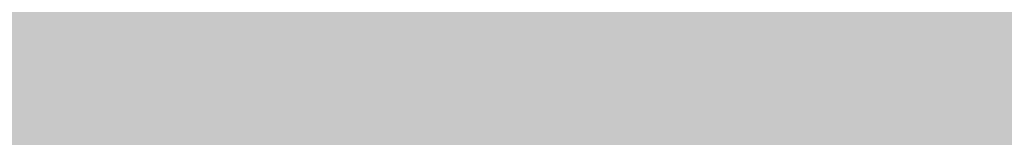
# Model space of a CAD drawing. Units: millimetres. Extents: x 0 to 2267, y 0 to 1823.
# Tile 203 of 256: x 1841.442 to 1842.748, y 1127.15 to 1127.306. Entities that reach past the tile are written whole.
import ezdxf

# ---------------------------------------------------------------- set-up
doc = ezdxf.new("R2010")
doc.units = ezdxf.units.MM
doc.header["$MEASUREMENT"] = 0
doc.layers.add('M-DIMS', color=2, linetype='Continuous', lineweight=25)
doc.layers.add('M-HATC', color=252, linetype='Continuous', lineweight=18)
doc.styles.get("Standard").update_dxf_attribs({"font": 'arial.ttf'})
doc.dimstyles.get("Standard").update_dxf_attribs({"dimtxt": 7, "dimasz": 4, "dimexe": 0.18, "dimexo": 0.0625, "dimgap": 0.09, "dimtad": 0, "dimdec": 0, "dimzin": 0, "dimdsep": 46, "dimtxsty": 'Standard', "dimcen": 0.09, "dimadec": 0, "dimazin": 0, "dimtfac": 1, "dimtdec": 0, "dimtofl": 0, "dimtmove": 0, "dimatfit": 3, "dimfxl": 1, "dimtolj": 1, "dimtzin": 0, "dimarcsym": 0})

# ---------------------------------------------------------------- blocks, each defined once
blk = doc.blocks.new('*D1')
at = {"layer": 'Defpoints', "color": 0, "transparency": 16777216}
for p in [(1593.4289, 1127.4171), (1843.4289, 1127.4171), (1843.4289, 955.6278)]:
    blk.add_point(p, dxfattribs=at)
at = {"layer": 'M-DIMS', "color": 0, "lineweight": -2, "transparency": 16777216}
for p, q in [((1593.4289, 1127.3546), (1593.4289, 955.4478)), ((1843.4289, 1127.3546), (1843.4289, 955.4478)), ((1597.4289, 955.6278), (1710.5582, 955.6278)), ((1839.4289, 955.6278), (1726.2996, 955.6278))]:
    blk.add_line(p, q, dxfattribs=at)
at = {"layer": 'M-DIMS', "color": 0, "transparency": 16777216}
for points in [[(1597.4289, 956.2944), (1597.4289, 954.9611), (1593.4289, 955.6278)], [(1839.4289, 956.2944), (1839.4289, 954.9611), (1843.4289, 955.6278)]]:
    blk.add_solid(points, dxfattribs=at)
at = {"layer": 'M-DIMS', "color": 0, "transparency": 16777216, "insert": (1718.4289, 955.6278), "char_height": 7, "attachment_point": 5}
blk.add_mtext('\\A1;250', dxfattribs=at)

msp = doc.modelspace()

# ---------------------------------------------------------------- hatches: boundary and pattern name
at = {"layer": 'M-HATC'}
h = msp.add_hatch(color=256, dxfattribs=at)
h.dxf.hatch_style = 1
h.paths.add_polyline_path([(2055.771, 1603.062), (1381.0868, 1603.062), (1381.0868, 1598.062), (2055.771, 1598.062)])
h.paths.add_polyline_path([(2055.771, 1598.062), (1381.0868, 1598.062), (1381.0868, 1593.062), (2055.771, 1593.062)])
h.paths.add_polyline_path([(2051.3074, 1536.7609), (1385.5504, 1536.7609), (1385.5504, 1526.7609), (1387.5504, 1526.7609), (1388.5366, 1525.0528), (1385.3319, 1521.2335), (1385.3319, 1521.2226), (2050.2542, 1522.7491), (2048.3212, 1525.0528), (2049.3074, 1526.7609), (2051.3074, 1526.7609)])
edge = h.paths.add_edge_path()
edge.add_arc((1847.5345, 1379.1492), 135, 222.603061, 222.890851, ccw=False)
edge.add_line((1748.1663, 1287.7656), (1683.0921, 1287.7656))
edge.add_arc((1583.7239, 1379.1492), 135, 317.109149, 317.396939, ccw=False)
edge.add_arc((1678.9686, 1290.6707), 5, 222.8909, 317.1091, ccw=False)
edge.add_arc((1774.2133, 1379.1492), 135, 222.603061, 222.890851, ccw=False)
edge.add_line((1674.8451, 1287.7656), (1609.7709, 1287.7656))
edge.add_arc((1510.4027, 1379.1492), 135, 317.109149, 317.396939, ccw=False)
edge.add_arc((1605.6474, 1290.6707), 5, 222.8909, 317.1091, ccw=False)
edge.add_arc((1700.8921, 1379.1492), 135, 222.603061, 222.890851, ccw=False)
edge.add_line((1601.5239, 1287.7656), (1536.4497, 1287.7656))
edge.add_arc((1437.0815, 1379.1492), 135, 317.109149, 317.396939, ccw=False)
edge.add_arc((1532.3262, 1290.6707), 5, 222.8909, 317.1091, ccw=False)
edge.add_arc((1627.5709, 1379.1492), 135, 222.603061, 222.890851, ccw=False)
edge.add_line((1528.2027, 1287.7656), (1505.9289, 1287.7656))
edge.add_spline(control_points=[(1505.9289, 1287.7656), (1504.2622, 1287.7656), (1504.2622, 1282.7656), (1505.9289, 1282.7656)], knot_values=[0, 0, 0, 0, 5, 5, 5, 5], degree=3, periodic=0)
edge.add_line((1505.9289, 1282.7656), (1930.9289, 1282.7656))
edge.add_spline(control_points=[(1930.9289, 1282.7656), (1932.5956, 1282.7656), (1932.5956, 1287.7656), (1930.9289, 1287.7656)], knot_values=[0, 0, 0, 0, 5, 5, 5, 5], degree=3, periodic=0)
edge.add_line((1930.9289, 1287.7656), (1903.0557, 1287.7656))
edge.add_arc((1803.6875, 1379.1492), 135, 317.109149, 317.396939, ccw=False)
edge.add_arc((1898.9322, 1290.6707), 5, 222.8909, 317.1091, ccw=False)
edge.add_arc((1994.1769, 1379.1492), 135, 222.603061, 222.890851, ccw=False)
edge.add_line((1894.8087, 1287.7656), (1829.7345, 1287.7656))
edge.add_arc((1730.3663, 1379.1492), 135, 317.109149, 317.396939, ccw=False)
edge.add_arc((1825.611, 1290.6707), 5, 222.8909, 317.1091, ccw=False)
edge.add_arc((1920.8557, 1379.1492), 135, 222.603061, 222.890851, ccw=False)
edge.add_line((1821.4875, 1287.7656), (1756.4133, 1287.7656))
edge.add_arc((1657.0451, 1379.1492), 135, 317.109149, 317.396939, ccw=False)
edge.add_arc((1752.2898, 1290.6707), 5, 222.8909, 317.1091, ccw=False)
edge = h.paths.add_edge_path()
edge.add_spline(control_points=[(1843.4289, 1227.2475), (1845.0956, 1227.2475), (1845.0956, 1232.2475), (1843.4289, 1232.2475)], knot_values=[0, 0, 0, 0, 5, 5, 5, 5], degree=3, periodic=0)
edge.add_line((1843.4289, 1232.2475), (1593.4289, 1232.2475))
edge.add_spline(control_points=[(1593.4289, 1232.2475), (1591.7622, 1232.2475), (1591.7622, 1227.2475), (1593.4289, 1227.2475)], knot_values=[0, 0, 0, 0, 5, 5, 5, 5], degree=3, periodic=0)
edge.add_line((1593.4289, 1227.2475), (1843.4289, 1227.2475))
h.paths.add_polyline_path([(1905.9289, 1127.4171), (1530.9289, 1127.4171, 0.414214), (1520.9289, 1117.4171), (1530.9289, 1117.4171), (1915.9289, 1117.4171, 0.414214)])
edge = h.paths.add_edge_path()
edge.add_arc((1397.0858, 1498.4078), 12.7299, 90.78215, 190.87871, ccw=False)
edge.add_line((1396.912, 1511.1365), (1428.0097, 1511.3488))
edge.add_line((1428.0097, 1511.3488), (1433.0097, 1511.3488))
edge.add_line((1433.0097, 1511.3488), (1434.439, 1511.3488))
edge.add_arc((1419.474, 1498.0804), 20, 41.561, 74.08211)
edge.add_line((1424.9592, 1517.3135), (1399.9351, 1517.2561))
edge.add_spline(control_points=[(1399.9307, 1517.2561), (1399.884, 1517.2131), (1399.8328, 1517.1689), (1399.7774, 1517.1236)], knot_values=[11.567499, 11.567499, 11.567499, 11.567499, 11.814249, 11.814249, 11.814249, 11.814249], degree=3, periodic=0)
edge.add_spline(control_points=[(1399.6328, 1517.0099), (1399.5831, 1516.9721), (1399.5307, 1516.9338), (1399.4759, 1516.8947)], knot_values=[11.167718, 11.167718, 11.167718, 11.167718, 11.365188, 11.365188, 11.365188, 11.365188], degree=3, periodic=0)
edge.add_spline(control_points=[(1399.3398, 1516.8001), (1399.1514, 1516.6719), (1398.9384, 1516.5377), (1398.704, 1516.3994)], knot_values=[10.376405, 10.376405, 10.376405, 10.376405, 11.00994, 11.00994, 11.00994, 11.00994], degree=3, periodic=0)
edge.add_spline(control_points=[(1398.6572, 1516.3719), (1398.5789, 1516.326), (1398.4983, 1516.2797), (1398.4155, 1516.2331)], knot_values=[10.125175, 10.125175, 10.125175, 10.125175, 10.334406, 10.334406, 10.334406, 10.334406], degree=3, periodic=0)
edge.add_spline(control_points=[(1398.2642, 1516.1487), (1398.196, 1516.1111), (1398.1263, 1516.0732), (1398.0555, 1516.0351)], knot_values=[9.832246, 9.832246, 9.832246, 9.832246, 9.999658, 9.999658, 9.999658, 9.999658], degree=3, periodic=0)
edge.add_spline(control_points=[(1397.9987, 1516.0048), (1397.7312, 1515.8621), (1397.446, 1515.7171), (1397.1466, 1515.5714)], knot_values=[9.161808, 9.161808, 9.161808, 9.161808, 9.787769, 9.787769, 9.787769, 9.787769], degree=3, periodic=0)
edge.add_spline(control_points=[(1397.1466, 1515.5714), (1396.8418, 1515.423), (1396.5222, 1515.274), (1396.1914, 1515.1262)], knot_values=[8.524455, 8.524455, 8.524455, 8.524455, 9.161808, 9.161808, 9.161808, 9.161808], degree=3, periodic=0)
edge.add_spline(control_points=[(1396.0777, 1515.0756), (1395.9854, 1515.0348), (1395.8922, 1514.994), (1395.7983, 1514.9534)], knot_values=[8.275193, 8.275193, 8.275193, 8.275193, 8.451726, 8.451726, 8.451726, 8.451726], degree=3, periodic=0)
edge.add_spline(control_points=[(1395.6018, 1514.8691), (1395.4997, 1514.8257), (1395.3968, 1514.7824), (1395.2932, 1514.7394)], knot_values=[7.962917, 7.962917, 7.962917, 7.962917, 8.152764, 8.152764, 8.152764, 8.152764], degree=3, periodic=0)
edge.add_spline(control_points=[(1395.2116, 1514.7057), (1394.8278, 1514.5475), (1394.4345, 1514.3929), (1394.0364, 1514.2442)], knot_values=[7.21254, 7.21254, 7.21254, 7.21254, 7.913148, 7.913148, 7.913148, 7.913148], degree=3, periodic=0)
edge.add_spline(control_points=[(1394.0364, 1514.2442), (1393.7076, 1514.1214), (1393.3754, 1514.0027), (1393.0427, 1513.8895)], knot_values=[6.633733, 6.633733, 6.633733, 6.633733, 7.21254, 7.21254, 7.21254, 7.21254], degree=3, periodic=0)
edge.add_spline(control_points=[(1392.8214, 1513.815), (1392.7198, 1513.7812), (1392.6181, 1513.7479), (1392.5166, 1513.7152)], knot_values=[6.328796, 6.328796, 6.328796, 6.328796, 6.505493, 6.505493, 6.505493, 6.505493], degree=3, periodic=0)
edge.add_spline(control_points=[(1392.5166, 1513.7152), (1392.3187, 1513.6515), (1392.1212, 1513.59), (1391.9244, 1513.531)], knot_values=[5.984605, 5.984605, 5.984605, 5.984605, 6.328796, 6.328796, 6.328796, 6.328796], degree=3, periodic=0)
edge.add_spline(control_points=[(1391.7915, 1513.4915), (1391.3122, 1513.3501), (1390.8384, 1513.2239), (1390.3784, 1513.1171)], knot_values=[5.066697, 5.066697, 5.066697, 5.066697, 5.907055, 5.907055, 5.907055, 5.907055], degree=3, periodic=0)
edge.add_spline(control_points=[(1390.3784, 1513.1171), (1390.1797, 1513.071), (1389.9836, 1513.0284), (1389.7907, 1512.9899)], knot_values=[4.70367, 4.70367, 4.70367, 4.70367, 5.066695, 5.066695, 5.066695, 5.066695], degree=3, periodic=0)
edge.add_spline(control_points=[(1389.422, 1512.9204), (1389.2459, 1512.8892), (1389.0729, 1512.8617), (1388.9036, 1512.8381)], knot_values=[4.130571, 4.130571, 4.130571, 4.130571, 4.469816, 4.469816, 4.469816, 4.469816], degree=3, periodic=0)
edge.add_spline(control_points=[(1388.9036, 1512.8381), (1388.591, 1512.7946), (1388.2911, 1512.7644), (1388.0071, 1512.7494)], knot_values=[3.504031, 3.504031, 3.504031, 3.504031, 4.130571, 4.130571, 4.130571, 4.130571], degree=3, periodic=0)
edge.add_spline(control_points=[(1387.9356, 1512.7459), (1387.8538, 1512.7423), (1387.7733, 1512.74), (1387.6944, 1512.739)], knot_values=[3.268866, 3.268866, 3.268866, 3.268866, 3.451164, 3.451164, 3.451164, 3.451164], degree=3, periodic=0)
edge.add_spline(control_points=[(1387.3351, 1512.7443), (1387.2076, 1512.7499), (1387.0847, 1512.7597), (1386.967, 1512.7739)], knot_values=[2.670686, 2.670686, 2.670686, 2.670686, 2.984, 2.984, 2.984, 2.984], degree=3, periodic=0)
edge.add_spline(control_points=[(1386.8327, 1512.7922), (1386.8209, 1512.7941), (1386.8092, 1512.7959), (1386.7975, 1512.7979)], knot_values=[2.516981, 2.516981, 2.516981, 2.516981, 2.549528, 2.549528, 2.549528, 2.549528], degree=3, periodic=0)
edge.add_spline(control_points=[(1386.4526, 1512.8735), (1386.4257, 1512.881), (1386.3993, 1512.889), (1386.3733, 1512.8972)], knot_values=[2.095869, 2.095869, 2.095869, 2.095869, 2.17941, 2.17941, 2.17941, 2.17941], degree=3, periodic=0)
edge.add_spline(control_points=[(1386.0691, 1513.0189), (1386.0634, 1513.0217), (1386.0577, 1513.0246), (1386.052, 1513.0275)], knot_values=[1.72453, 1.72453, 1.72453, 1.72453, 1.745933, 1.745933, 1.745933, 1.745933], degree=3, periodic=0)
edge.add_arc((1399.474, 1498.0804), 20, 131.82432, 180)
edge.add_arc((1630.3336, 1505.5484), 250.9708, 181.705176, 236.427975)
edge.add_arc((1605.3399, 1483.3044), 218.7822, 238.660829, 243.34961)
edge.add_arc((1647.0911, 1510.3592), 262.8986, 183.129836, 237.853442, ccw=False)
h.paths.add_polyline_path([(1406.5369, 1391.9644, 0.149382), (1491.5506, 1296.4418, -0.129517)], flags=17)
edge = h.paths.add_edge_path()
edge.add_arc((2037.3838, 1498.0804), 20, 0, 48.26587)
edge.add_spline(control_points=[(2050.6973, 1513.0052), (2050.6512, 1512.9847), (2050.6034, 1512.9655), (2050.5539, 1512.9477)], knot_values=[1.835652, 1.835652, 1.835652, 1.835652, 2.000781, 2.000781, 2.000781, 2.000781], degree=3, periodic=0)
edge.add_spline(control_points=[(2050.4616, 1512.9166), (2050.479, 1512.9221), (2050.4963, 1512.9277), (2050.5133, 1512.9335)], knot_values=[2.045477, 2.045477, 2.045477, 2.045477, 2.101389, 2.101389, 2.101389, 2.101389], degree=3, periodic=0)
edge.add_spline(control_points=[(2050.129, 1512.8342), (2050.1984, 1512.8473), (2050.2657, 1512.8623), (2050.3308, 1512.8792)], knot_values=[2.237629, 2.237629, 2.237629, 2.237629, 2.435841, 2.435841, 2.435841, 2.435841], degree=3, periodic=0)
edge.add_spline(control_points=[(2050.0946, 1512.8278), (2050.1061, 1512.8299), (2050.1176, 1512.832), (2050.129, 1512.8342)], knot_values=[2.435841, 2.435841, 2.435841, 2.435841, 2.468321, 2.468321, 2.468321, 2.468321], degree=3, periodic=0)
edge.add_spline(control_points=[(2049.7843, 1512.7851), (2049.8552, 1512.7922), (2049.9243, 1512.8008), (2049.9917, 1512.8109)], knot_values=[2.563852, 2.563852, 2.563852, 2.563852, 2.748541, 2.748541, 2.748541, 2.748541], degree=3, periodic=0)
edge.add_spline(control_points=[(2049.4052, 1512.7617), (2049.5364, 1512.7653), (2049.6629, 1512.773), (2049.7843, 1512.7851)], knot_values=[2.748541, 2.748541, 2.748541, 2.748541, 3.064882, 3.064882, 3.064882, 3.064882], degree=3, periodic=0)
edge.add_spline(control_points=[(2049.1698, 1512.7597), (2049.2336, 1512.7591), (2049.2965, 1512.7594), (2049.3584, 1512.7606)], knot_values=[3.102309, 3.102309, 3.102309, 3.102309, 3.2503, 3.2503, 3.2503, 3.2503], degree=3, periodic=0)
edge.add_spline(control_points=[(2048.8573, 1512.7691), (2048.9638, 1512.7638), (2049.068, 1512.7606), (2049.1698, 1512.7597)], knot_values=[3.2503, 3.2503, 3.2503, 3.2503, 3.486069, 3.486069, 3.486069, 3.486069], degree=3, periodic=0)
edge.add_spline(control_points=[(2048.6924, 1512.7789), (2048.3729, 1512.8009), (2048.0345, 1512.8411), (2047.6817, 1512.897)], knot_values=[3.606429, 3.606429, 3.606429, 3.606429, 4.2989, 4.2989, 4.2989, 4.2989], degree=3, periodic=0)
edge.add_spline(control_points=[(2047.6817, 1512.897), (2047.5458, 1512.9185), (2047.4077, 1512.9424), (2047.2678, 1512.9685)], knot_values=[4.2989, 4.2989, 4.2989, 4.2989, 4.565769, 4.565769, 4.565769, 4.565769], degree=3, periodic=0)
edge.add_spline(control_points=[(2047.2678, 1512.9685), (2047.1449, 1512.9914), (2047.0207, 1513.016), (2046.8951, 1513.0422)], knot_values=[4.565769, 4.565769, 4.565769, 4.565769, 4.799971, 4.799971, 4.799971, 4.799971], degree=3, periodic=0)
edge.add_spline(control_points=[(2046.8951, 1513.0422), (2046.5286, 1513.1188), (2046.1513, 1513.209), (2045.7676, 1513.3107)], knot_values=[4.799971, 4.799971, 4.799971, 4.799971, 5.483718, 5.483718, 5.483718, 5.483718], degree=3, periodic=0)
edge.add_spline(control_points=[(2045.7676, 1513.3107), (2045.3724, 1513.4154), (2044.9704, 1513.5322), (2044.5662, 1513.6588)], knot_values=[5.483718, 5.483718, 5.483718, 5.483718, 6.187866, 6.187866, 6.187866, 6.187866], degree=3, periodic=0)
edge.add_spline(control_points=[(2044.5662, 1513.6588), (2044.4149, 1513.7061), (2044.2633, 1513.7549), (2044.1116, 1513.8048)], knot_values=[6.187866, 6.187866, 6.187866, 6.187866, 6.451551, 6.451551, 6.451551, 6.451551], degree=3, periodic=0)
edge.add_spline(control_points=[(2044.1116, 1513.8048), (2043.9967, 1513.8427), (2043.8817, 1513.8813), (2043.7668, 1513.9205)], knot_values=[6.451551, 6.451551, 6.451551, 6.451551, 6.651434, 6.651434, 6.651434, 6.651434], degree=3, periodic=0)
edge.add_spline(control_points=[(2043.7668, 1513.9205), (2043.3716, 1514.0554), (2042.9774, 1514.1979), (2042.5886, 1514.3458)], knot_values=[6.651434, 6.651434, 6.651434, 6.651434, 7.338879, 7.338879, 7.338879, 7.338879], degree=3, periodic=0)
edge.add_spline(control_points=[(2042.5886, 1514.3458), (2042.1643, 1514.5071), (2041.7465, 1514.6749), (2041.3409, 1514.846)], knot_values=[7.338879, 7.338879, 7.338879, 7.338879, 8.089209, 8.089209, 8.089209, 8.089209], degree=3, periodic=0)
edge.add_spline(control_points=[(2041.3409, 1514.846), (2041.1028, 1514.9465), (2040.869, 1515.0481), (2040.6405, 1515.1502)], knot_values=[8.089209, 8.089209, 8.089209, 8.089209, 8.529587, 8.529587, 8.529587, 8.529587], degree=3, periodic=0)
edge.add_spline(control_points=[(2040.51, 1515.2089), (2040.0824, 1515.4022), (2039.6747, 1515.5971), (2039.295, 1515.7894)], knot_values=[8.613818, 8.613818, 8.613818, 8.613818, 9.44571, 9.44571, 9.44571, 9.44571], degree=3, periodic=0)
edge.add_spline(control_points=[(2039.295, 1515.7894), (2039.0618, 1515.9075), (2038.8391, 1516.0246), (2038.6288, 1516.1398)], knot_values=[9.44571, 9.44571, 9.44571, 9.44571, 9.956404, 9.956404, 9.956404, 9.956404], degree=3, periodic=0)
edge.add_spline(control_points=[(2038.6288, 1516.1398), (2038.5187, 1516.2001), (2038.4121, 1516.2598), (2038.309, 1516.3189)], knot_values=[9.956404, 9.956404, 9.956404, 9.956404, 10.223542, 10.223542, 10.223542, 10.223542], degree=3, periodic=0)
edge.add_spline(control_points=[(2038.309, 1516.3189), (2038.2138, 1516.3735), (2038.1216, 1516.4276), (2038.0328, 1516.481)], knot_values=[10.223542, 10.223542, 10.223542, 10.223542, 10.47051, 10.47051, 10.47051, 10.47051], degree=3, periodic=0)
edge.add_spline(control_points=[(2038.0328, 1516.481), (2037.7855, 1516.6296), (2037.5639, 1516.773), (2037.3722, 1516.909)], knot_values=[10.47051, 10.47051, 10.47051, 10.47051, 11.15767, 11.15767, 11.15767, 11.15767], degree=3, periodic=0)
edge.add_spline(control_points=[(2037.3722, 1516.909), (2037.2789, 1516.9752), (2037.1927, 1517.0396), (2037.1142, 1517.102)], knot_values=[11.15767, 11.15767, 11.15767, 11.15767, 11.49227, 11.49227, 11.49227, 11.49227], degree=3, periodic=0)
edge.add_spline(control_points=[(2036.8564, 1517.3259), (2036.9148, 1517.2692), (2036.9814, 1517.2103), (2037.0557, 1517.1492)], knot_values=[11.577341, 11.577341, 11.577341, 11.577341, 11.91035, 11.91035, 11.91035, 11.91035], degree=3, periodic=0)
edge.add_spline(control_points=[(2036.8074, 1517.3748), (2036.823, 1517.3587), (2036.8393, 1517.3424), (2036.8564, 1517.3259)], knot_values=[11.91035, 11.91035, 11.91035, 11.91035, 12.007402, 12.007402, 12.007402, 12.007402], degree=3, periodic=0)
edge.add_spline(control_points=[(2036.7017, 1517.494), (2036.7104, 1517.483), (2036.7196, 1517.4719), (2036.7291, 1517.4606)], knot_values=[12.184155, 12.184155, 12.184155, 12.184155, 12.255409, 12.255409, 12.255409, 12.255409], degree=3, periodic=0)
edge.add_spline(control_points=[(2036.6159, 1517.6205), (2036.62, 1517.613), (2036.6243, 1517.6055), (2036.6289, 1517.5979)], knot_values=[12.487913, 12.487913, 12.487913, 12.487913, 12.541035, 12.541035, 12.541035, 12.541035], degree=3, periodic=0)
edge.add_spline(control_points=[(2036.5635, 1517.786), (2036.5637, 1517.7794), (2036.5642, 1517.7726), (2036.565, 1517.7658)], knot_values=[12.911761, 12.911761, 12.911761, 12.911761, 12.968286, 12.968286, 12.968286, 12.968286], degree=3, periodic=0)
edge.add_spline(control_points=[(2036.6166, 1517.9304), (2036.6125, 1517.9259), (2036.6086, 1517.9212), (2036.6049, 1517.9165)], knot_values=[13.382527, 13.382527, 13.382527, 13.382527, 13.433791, 13.433791, 13.433791, 13.433791], degree=3, periodic=0)
edge.add_spline(control_points=[(2036.749, 1518.017), (2036.7361, 1518.0116), (2036.7239, 1518.006), (2036.7124, 1518.0002)], knot_values=[13.726299, 13.726299, 13.726299, 13.726299, 13.809928, 13.809928, 13.809928, 13.809928], degree=3, periodic=0)
edge.add_spline(control_points=[(2036.8604, 1518.0528), (2036.8386, 1518.0474), (2036.8181, 1518.0416), (2036.7988, 1518.0353)], knot_values=[13.910887, 13.910887, 13.910887, 13.910887, 14.02153, 14.02153, 14.02153, 14.02153], degree=3, periodic=0)
edge.add_line((2036.9639, 1518.0804), (2032.3838, 1518.0804))
edge.add_line((2032.3838, 1518.0804), (2027.3838, 1518.0804))
edge.add_line((2027.3838, 1518.0804), (2022.3838, 1518.0804))
edge.add_line((2022.3838, 1518.0804), (2017.3838, 1518.0804))
edge.add_arc((2017.3838, 1498.0804), 20, 90, 138.439)
edge.add_line((2002.4188, 1511.3488), (2003.8481, 1511.3488))
edge.add_line((2003.8481, 1511.3488), (2008.8481, 1511.3488))
edge.add_line((2008.8481, 1511.3488), (2039.772, 1511.1377))
edge.add_arc((2039.772, 1498.4078), 12.7299, -10.87871, 90, ccw=False)
edge.add_arc((1789.7668, 1510.3592), 262.8986, 302.146558, 356.870164, ccw=False)
edge.add_arc((1831.5179, 1483.3044), 218.7822, 296.65039, 301.339171)
edge.add_arc((1806.5242, 1505.5484), 250.9708, 303.572025, 358.294824)
h.paths.add_polyline_path([(2030.321, 1391.9644, -0.129517), (1945.3072, 1296.4418, 0.149382)], flags=17)
edge = h.paths.add_edge_path()
edge.add_spline(control_points=[(2037.2464, 1518.0821), (2037.2898, 1518.081), (2037.3355, 1518.0804), (2037.3838, 1518.0804)], knot_values=[0.000012, 0.000012, 0.000012, 0.000012, 0.144754, 0.144754, 0.144754, 0.144754], degree=3, periodic=0)
edge.add_line((2037.3357, 1518.0804), (2037.0096, 1518.0804))
edge.add_spline(control_points=[(2037.0096, 1518.0804), (2036.9822, 1518.0768), (2036.956, 1518.0727), (2036.9312, 1518.0681)], knot_values=[14.13465, 14.13465, 14.13465, 14.13465, 14.247197, 14.247197, 14.247197, 14.247197], degree=3, periodic=0)
edge.add_spline(control_points=[(2036.9312, 1518.0681), (2036.9276, 1518.0674), (2036.9241, 1518.0667), (2036.9205, 1518.0661)], knot_values=[14.118315, 14.118315, 14.118315, 14.118315, 14.13465, 14.13465, 14.13465, 14.13465], degree=3, periodic=0)
edge.add_spline(control_points=[(2036.9205, 1518.0661), (2036.9118, 1518.0644), (2036.9032, 1518.0626), (2036.8948, 1518.0608)], knot_values=[14.078086, 14.078086, 14.078086, 14.078086, 14.118315, 14.118315, 14.118315, 14.118315], degree=3, periodic=0)
edge.add_spline(control_points=[(2036.8948, 1518.0608), (2036.883, 1518.0583), (2036.8716, 1518.0556), (2036.8604, 1518.0528)], knot_values=[14.02153, 14.02153, 14.02153, 14.02153, 14.078086, 14.078086, 14.078086, 14.078086], degree=3, periodic=0)
edge.add_spline(control_points=[(2036.8604, 1518.0528), (2036.8386, 1518.0474), (2036.8181, 1518.0416), (2036.7988, 1518.0353)], knot_values=[13.910887, 13.910887, 13.910887, 13.910887, 14.02153, 14.02153, 14.02153, 14.02153], degree=3, periodic=0)
edge.add_spline(control_points=[(2036.7988, 1518.0353), (2036.7981, 1518.035), (2036.7974, 1518.0348), (2036.7967, 1518.0346)], knot_values=[13.906906, 13.906906, 13.906906, 13.906906, 13.910887, 13.910887, 13.910887, 13.910887], degree=3, periodic=0)
edge.add_spline(control_points=[(2036.7967, 1518.0346), (2036.7882, 1518.0318), (2036.7799, 1518.0289), (2036.7719, 1518.0259)], knot_values=[13.857826, 13.857826, 13.857826, 13.857826, 13.906906, 13.906906, 13.906906, 13.906906], degree=3, periodic=0)
edge.add_spline(control_points=[(2036.7719, 1518.0259), (2036.764, 1518.023), (2036.7564, 1518.02), (2036.749, 1518.017)], knot_values=[13.809928, 13.809928, 13.809928, 13.809928, 13.857826, 13.857826, 13.857826, 13.857826], degree=3, periodic=0)
edge.add_spline(control_points=[(2036.749, 1518.017), (2036.7361, 1518.0116), (2036.7239, 1518.006), (2036.7124, 1518.0002)], knot_values=[13.726299, 13.726299, 13.726299, 13.726299, 13.809928, 13.809928, 13.809928, 13.809928], degree=3, periodic=0)
edge.add_spline(control_points=[(2036.7124, 1518.0002), (2036.7121, 1518), (2036.7118, 1517.9999), (2036.7115, 1517.9997)], knot_values=[13.723993, 13.723993, 13.723993, 13.723993, 13.726299, 13.726299, 13.726299, 13.726299], degree=3, periodic=0)
edge.add_spline(control_points=[(2036.7115, 1517.9997), (2036.7063, 1517.9971), (2036.7013, 1517.9944), (2036.6965, 1517.9917)], knot_values=[13.686536, 13.686536, 13.686536, 13.686536, 13.723993, 13.723993, 13.723993, 13.723993], degree=3, periodic=0)
edge.add_spline(control_points=[(2036.6965, 1517.9917), (2036.6919, 1517.9891), (2036.6874, 1517.9865), (2036.6831, 1517.9839)], knot_values=[13.651251, 13.651251, 13.651251, 13.651251, 13.686536, 13.686536, 13.686536, 13.686536], degree=3, periodic=0)
edge.add_spline(control_points=[(2036.6831, 1517.9839), (2036.6764, 1517.9798), (2036.67, 1517.9757), (2036.6639, 1517.9714)], knot_values=[13.596804, 13.596804, 13.596804, 13.596804, 13.651251, 13.651251, 13.651251, 13.651251], degree=3, periodic=0)
edge.add_spline(control_points=[(2036.6639, 1517.9714), (2036.6636, 1517.9712), (2036.6633, 1517.9709), (2036.6629, 1517.9707)], knot_values=[13.593956, 13.593956, 13.593956, 13.593956, 13.596804, 13.596804, 13.596804, 13.596804], degree=3, periodic=0)
edge.add_spline(control_points=[(2036.6629, 1517.9707), (2036.6603, 1517.9689), (2036.6577, 1517.967), (2036.6552, 1517.9651)], knot_values=[13.570322, 13.570322, 13.570322, 13.570322, 13.593956, 13.593956, 13.593956, 13.593956], degree=3, periodic=0)
edge.add_spline(control_points=[(2036.6552, 1517.9651), (2036.6525, 1517.9631), (2036.6499, 1517.9611), (2036.6474, 1517.9591)], knot_values=[13.545477, 13.545477, 13.545477, 13.545477, 13.570322, 13.570322, 13.570322, 13.570322], degree=3, periodic=0)
edge.add_spline(control_points=[(2036.6474, 1517.9591), (2036.6472, 1517.9589), (2036.6471, 1517.9588), (2036.6469, 1517.9587)], knot_values=[13.543931, 13.543931, 13.543931, 13.543931, 13.545477, 13.545477, 13.545477, 13.545477], degree=3, periodic=0)
edge.add_spline(control_points=[(2036.6469, 1517.9587), (2036.6412, 1517.9541), (2036.6358, 1517.9494), (2036.6307, 1517.9447)], knot_values=[13.488237, 13.488237, 13.488237, 13.488237, 13.543931, 13.543931, 13.543931, 13.543931], degree=3, periodic=0)
edge.add_spline(control_points=[(2036.6307, 1517.9447), (2036.6282, 1517.9423), (2036.6257, 1517.9399), (2036.6233, 1517.9374)], knot_values=[13.460307, 13.460307, 13.460307, 13.460307, 13.488237, 13.488237, 13.488237, 13.488237], degree=3, periodic=0)
edge.add_spline(control_points=[(2036.6233, 1517.9374), (2036.6215, 1517.9356), (2036.6198, 1517.9338), (2036.6181, 1517.932)], knot_values=[13.439712, 13.439712, 13.439712, 13.439712, 13.460307, 13.460307, 13.460307, 13.460307], degree=3, periodic=0)
edge.add_spline(control_points=[(2036.6181, 1517.932), (2036.6176, 1517.9315), (2036.6171, 1517.9309), (2036.6166, 1517.9304)], knot_values=[13.433791, 13.433791, 13.433791, 13.433791, 13.439712, 13.439712, 13.439712, 13.439712], degree=3, periodic=0)
edge.add_spline(control_points=[(2036.6166, 1517.9304), (2036.6125, 1517.9259), (2036.6086, 1517.9212), (2036.6049, 1517.9165)], knot_values=[13.382527, 13.382527, 13.382527, 13.382527, 13.433791, 13.433791, 13.433791, 13.433791], degree=3, periodic=0)
edge.add_spline(control_points=[(2036.6049, 1517.9165), (2036.6026, 1517.9135), (2036.6004, 1517.9104), (2036.5982, 1517.9074)], knot_values=[13.350017, 13.350017, 13.350017, 13.350017, 13.382527, 13.382527, 13.382527, 13.382527], degree=3, periodic=0)
edge.add_spline(control_points=[(2036.5982, 1517.9074), (2036.5972, 1517.9059), (2036.5962, 1517.9043), (2036.5952, 1517.9028)], knot_values=[13.333922, 13.333922, 13.333922, 13.333922, 13.350017, 13.350017, 13.350017, 13.350017], degree=3, periodic=0)
edge.add_spline(control_points=[(2036.5952, 1517.9028), (2036.5945, 1517.9018), (2036.5939, 1517.9009), (2036.5933, 1517.8999)], knot_values=[13.323828, 13.323828, 13.323828, 13.323828, 13.333922, 13.333922, 13.333922, 13.333922], degree=3, periodic=0)
edge.add_spline(control_points=[(2036.5933, 1517.8999), (2036.5905, 1517.8955), (2036.5879, 1517.8909), (2036.5855, 1517.8864)], knot_values=[13.277545, 13.277545, 13.277545, 13.277545, 13.323828, 13.323828, 13.323828, 13.323828], degree=3, periodic=0)
edge.add_spline(control_points=[(2036.5855, 1517.8864), (2036.5836, 1517.8827), (2036.5817, 1517.8789), (2036.5801, 1517.8751)], knot_values=[13.240119, 13.240119, 13.240119, 13.240119, 13.277545, 13.277545, 13.277545, 13.277545], degree=3, periodic=0)
edge.add_spline(control_points=[(2036.5801, 1517.8751), (2036.5795, 1517.8739), (2036.579, 1517.8727), (2036.5785, 1517.8715)], knot_values=[13.228211, 13.228211, 13.228211, 13.228211, 13.240119, 13.240119, 13.240119, 13.240119], degree=3, periodic=0)
edge.add_spline(control_points=[(2036.5785, 1517.8715), (2036.578, 1517.8702), (2036.5774, 1517.869), (2036.5769, 1517.8677)], knot_values=[13.215717, 13.215717, 13.215717, 13.215717, 13.228211, 13.228211, 13.228211, 13.228211], degree=3, periodic=0)
edge.add_spline(control_points=[(2036.5769, 1517.8677), (2036.5755, 1517.864), (2036.5741, 1517.8603), (2036.5729, 1517.8565)], knot_values=[13.179847, 13.179847, 13.179847, 13.179847, 13.215717, 13.215717, 13.215717, 13.215717], degree=3, periodic=0)
edge.add_spline(control_points=[(2036.5729, 1517.8565), (2036.5713, 1517.8515), (2036.5699, 1517.8464), (2036.5687, 1517.8413)], knot_values=[13.132017, 13.132017, 13.132017, 13.132017, 13.179847, 13.179847, 13.179847, 13.179847], degree=3, periodic=0)
edge.add_spline(control_points=[(2036.5687, 1517.8413), (2036.5684, 1517.8402), (2036.5682, 1517.8392), (2036.568, 1517.8382)], knot_values=[13.122482, 13.122482, 13.122482, 13.122482, 13.132017, 13.132017, 13.132017, 13.132017], degree=3, periodic=0)
edge.add_spline(control_points=[(2036.568, 1517.8382), (2036.5676, 1517.8363), (2036.5672, 1517.8345), (2036.5669, 1517.8327)], knot_values=[13.105592, 13.105592, 13.105592, 13.105592, 13.122482, 13.122482, 13.122482, 13.122482], degree=3, periodic=0)
edge.add_spline(control_points=[(2036.5669, 1517.8327), (2036.5662, 1517.8292), (2036.5657, 1517.8257), (2036.5652, 1517.8222)], knot_values=[13.074063, 13.074063, 13.074063, 13.074063, 13.105592, 13.105592, 13.105592, 13.105592], degree=3, periodic=0)
edge.add_spline(control_points=[(2036.5652, 1517.8222), (2036.5652, 1517.8222), (2036.5652, 1517.8222), (2036.5652, 1517.8222)], knot_values=[13.074043, 13.074043, 13.074043, 13.074043, 13.074063, 13.074063, 13.074063, 13.074063], degree=3, periodic=0)
edge.add_spline(control_points=[(2036.5652, 1517.8222), (2036.5644, 1517.8164), (2036.5639, 1517.8106), (2036.5636, 1517.8046)], knot_values=[13.021884, 13.021884, 13.021884, 13.021884, 13.074043, 13.074043, 13.074043, 13.074043], degree=3, periodic=0)
edge.add_spline(control_points=[(2036.5636, 1517.8046), (2036.5636, 1517.804), (2036.5636, 1517.8034), (2036.5635, 1517.8028)], knot_values=[13.01674, 13.01674, 13.01674, 13.01674, 13.021884, 13.021884, 13.021884, 13.021884], degree=3, periodic=0)
edge.add_spline(control_points=[(2036.5635, 1517.8028), (2036.5634, 1517.8005), (2036.5634, 1517.7982), (2036.5634, 1517.7958)], knot_values=[12.996438, 12.996438, 12.996438, 12.996438, 13.01674, 13.01674, 13.01674, 13.01674], degree=3, periodic=0)
edge.add_spline(control_points=[(2036.5634, 1517.7958), (2036.5633, 1517.7926), (2036.5634, 1517.7893), (2036.5635, 1517.786)], knot_values=[12.968286, 12.968286, 12.968286, 12.968286, 12.996438, 12.996438, 12.996438, 12.996438], degree=3, periodic=0)
edge.add_spline(control_points=[(2036.5635, 1517.786), (2036.5637, 1517.7794), (2036.5642, 1517.7726), (2036.565, 1517.7658)], knot_values=[12.911761, 12.911761, 12.911761, 12.911761, 12.968286, 12.968286, 12.968286, 12.968286], degree=3, periodic=0)
edge.add_spline(control_points=[(2036.565, 1517.7658), (2036.565, 1517.7657), (2036.565, 1517.7656), (2036.565, 1517.7656)], knot_values=[12.911017, 12.911017, 12.911017, 12.911017, 12.911761, 12.911761, 12.911761, 12.911761], degree=3, periodic=0)
edge.add_spline(control_points=[(2036.565, 1517.7656), (2036.5654, 1517.7625), (2036.5658, 1517.7593), (2036.5663, 1517.7562)], knot_values=[12.88528, 12.88528, 12.88528, 12.88528, 12.911017, 12.911017, 12.911017, 12.911017], degree=3, periodic=0)
edge.add_spline(control_points=[(2036.5663, 1517.7562), (2036.5667, 1517.7534), (2036.5672, 1517.7506), (2036.5677, 1517.7478)], knot_values=[12.862519, 12.862519, 12.862519, 12.862519, 12.88528, 12.88528, 12.88528, 12.88528], degree=3, periodic=0)
edge.add_spline(control_points=[(2036.5677, 1517.7478), (2036.5678, 1517.7474), (2036.5679, 1517.7469), (2036.568, 1517.7465)], knot_values=[12.858885, 12.858885, 12.858885, 12.858885, 12.862519, 12.862519, 12.862519, 12.862519], degree=3, periodic=0)
edge.add_spline(control_points=[(2036.568, 1517.7465), (2036.5692, 1517.7399), (2036.5707, 1517.7332), (2036.5724, 1517.7264)], knot_values=[12.8053, 12.8053, 12.8053, 12.8053, 12.858885, 12.858885, 12.858885, 12.858885], degree=3, periodic=0)
edge.add_spline(control_points=[(2036.5724, 1517.7264), (2036.5734, 1517.7226), (2036.5745, 1517.7187), (2036.5756, 1517.7149)], knot_values=[12.775176, 12.775176, 12.775176, 12.775176, 12.8053, 12.8053, 12.8053, 12.8053], degree=3, periodic=0)
edge.add_spline(control_points=[(2036.5756, 1517.7149), (2036.5763, 1517.7125), (2036.577, 1517.7102), (2036.5778, 1517.7078)], knot_values=[12.756759, 12.756759, 12.756759, 12.756759, 12.775176, 12.775176, 12.775176, 12.775176], degree=3, periodic=0)
edge.add_spline(control_points=[(2036.5778, 1517.7078), (2036.5781, 1517.7067), (2036.5784, 1517.7057), (2036.5787, 1517.7047)], knot_values=[12.748742, 12.748742, 12.748742, 12.748742, 12.756759, 12.756759, 12.756759, 12.756759], degree=3, periodic=0)
edge.add_spline(control_points=[(2036.5787, 1517.7047), (2036.5808, 1517.6983), (2036.5831, 1517.6919), (2036.5856, 1517.6854)], knot_values=[12.69959, 12.69959, 12.69959, 12.69959, 12.748742, 12.748742, 12.748742, 12.748742], degree=3, periodic=0)
edge.add_spline(control_points=[(2036.5856, 1517.6854), (2036.5876, 1517.68), (2036.5898, 1517.6746), (2036.5921, 1517.6692)], knot_values=[12.659038, 12.659038, 12.659038, 12.659038, 12.69959, 12.69959, 12.69959, 12.69959], degree=3, periodic=0)
edge.add_spline(control_points=[(2036.5921, 1517.6692), (2036.594, 1517.6648), (2036.5959, 1517.6605), (2036.5979, 1517.6561)], knot_values=[12.626806, 12.626806, 12.626806, 12.626806, 12.659038, 12.659038, 12.659038, 12.659038], degree=3, periodic=0)
edge.add_spline(control_points=[(2036.5979, 1517.6561), (2036.5984, 1517.6551), (2036.5989, 1517.6541), (2036.5993, 1517.6531)], knot_values=[12.619394, 12.619394, 12.619394, 12.619394, 12.626806, 12.626806, 12.626806, 12.626806], degree=3, periodic=0)
edge.add_spline(control_points=[(2036.5993, 1517.6531), (2036.6043, 1517.6424), (2036.6099, 1517.6315), (2036.6159, 1517.6205)], knot_values=[12.541039, 12.541039, 12.541039, 12.541039, 12.619394, 12.619394, 12.619394, 12.619394], degree=3, periodic=0)
edge.add_spline(control_points=[(2036.6159, 1517.6205), (2036.6159, 1517.6205), (2036.6159, 1517.6205), (2036.6159, 1517.6205)], knot_values=[12.541035, 12.541035, 12.541035, 12.541035, 12.541039, 12.541039, 12.541039, 12.541039], degree=3, periodic=0)
edge.add_spline(control_points=[(2036.6159, 1517.6205), (2036.62, 1517.613), (2036.6243, 1517.6055), (2036.6289, 1517.5979)], knot_values=[12.487913, 12.487913, 12.487913, 12.487913, 12.541035, 12.541035, 12.541035, 12.541035], degree=3, periodic=0)
edge.add_spline(control_points=[(2036.6289, 1517.5979), (2036.6326, 1517.5916), (2036.6365, 1517.5853), (2036.6406, 1517.5789)], knot_values=[12.443982, 12.443982, 12.443982, 12.443982, 12.487913, 12.487913, 12.487913, 12.487913], degree=3, periodic=0)
edge.add_spline(control_points=[(2036.6406, 1517.5789), (2036.6414, 1517.5776), (2036.6423, 1517.5763), (2036.6431, 1517.5749)], knot_values=[12.434996, 12.434996, 12.434996, 12.434996, 12.443982, 12.443982, 12.443982, 12.443982], degree=3, periodic=0)
edge.add_spline(control_points=[(2036.6431, 1517.5749), (2036.6531, 1517.5596), (2036.6639, 1517.5439), (2036.6756, 1517.528)], knot_values=[12.329647, 12.329647, 12.329647, 12.329647, 12.434996, 12.434996, 12.434996, 12.434996], degree=3, periodic=0)
edge.add_spline(control_points=[(2036.6756, 1517.528), (2036.6839, 1517.5168), (2036.6925, 1517.5055), (2036.7017, 1517.494)], knot_values=[12.255409, 12.255409, 12.255409, 12.255409, 12.329647, 12.329647, 12.329647, 12.329647], degree=3, periodic=0)
edge.add_spline(control_points=[(2036.7017, 1517.494), (2036.7104, 1517.483), (2036.7196, 1517.4719), (2036.7291, 1517.4606)], knot_values=[12.184155, 12.184155, 12.184155, 12.184155, 12.255409, 12.255409, 12.255409, 12.255409], degree=3, periodic=0)
edge.add_spline(control_points=[(2036.7291, 1517.4606), (2036.7436, 1517.4435), (2036.759, 1517.4262), (2036.7753, 1517.4085)], knot_values=[12.075961, 12.075961, 12.075961, 12.075961, 12.184155, 12.184155, 12.184155, 12.184155], degree=3, periodic=0)
edge.add_spline(control_points=[(2036.7753, 1517.4085), (2036.7763, 1517.4075), (2036.7773, 1517.4064), (2036.7783, 1517.4054)], knot_values=[12.069502, 12.069502, 12.069502, 12.069502, 12.075961, 12.075961, 12.075961, 12.075961], degree=3, periodic=0)
edge.add_spline(control_points=[(2036.7783, 1517.4054), (2036.7877, 1517.3953), (2036.7974, 1517.385), (2036.8074, 1517.3748)], knot_values=[12.007402, 12.007402, 12.007402, 12.007402, 12.069502, 12.069502, 12.069502, 12.069502], degree=3, periodic=0)
edge.add_spline(control_points=[(2036.8074, 1517.3748), (2036.823, 1517.3587), (2036.8393, 1517.3424), (2036.8564, 1517.3259)], knot_values=[11.91035, 11.91035, 11.91035, 11.91035, 12.007402, 12.007402, 12.007402, 12.007402], degree=3, periodic=0)
edge.add_spline(control_points=[(2036.8564, 1517.3259), (2036.9148, 1517.2692), (2036.9814, 1517.2103), (2037.0557, 1517.1492)], knot_values=[11.577341, 11.577341, 11.577341, 11.577341, 11.91035, 11.91035, 11.91035, 11.91035], degree=3, periodic=0)
edge.add_spline(control_points=[(2037.0557, 1517.1492), (2037.0747, 1517.1336), (2037.0942, 1517.1179), (2037.1142, 1517.102)], knot_values=[11.49227, 11.49227, 11.49227, 11.49227, 11.577341, 11.577341, 11.577341, 11.577341], degree=3, periodic=0)
edge.add_spline(control_points=[(2037.1142, 1517.102), (2037.1927, 1517.0396), (2037.2789, 1516.9752), (2037.3722, 1516.909)], knot_values=[11.15767, 11.15767, 11.15767, 11.15767, 11.49227, 11.49227, 11.49227, 11.49227], degree=3, periodic=0)
edge.add_spline(control_points=[(2037.3722, 1516.909), (2037.5639, 1516.773), (2037.7855, 1516.6296), (2038.0328, 1516.481)], knot_values=[10.47051, 10.47051, 10.47051, 10.47051, 11.15767, 11.15767, 11.15767, 11.15767], degree=3, periodic=0)
edge.add_spline(control_points=[(2038.0328, 1516.481), (2038.1216, 1516.4276), (2038.2138, 1516.3735), (2038.309, 1516.3189)], knot_values=[10.223542, 10.223542, 10.223542, 10.223542, 10.47051, 10.47051, 10.47051, 10.47051], degree=3, periodic=0)
edge.add_spline(control_points=[(2038.309, 1516.3189), (2038.4121, 1516.2598), (2038.5187, 1516.2001), (2038.6288, 1516.1398)], knot_values=[9.956404, 9.956404, 9.956404, 9.956404, 10.223542, 10.223542, 10.223542, 10.223542], degree=3, periodic=0)
edge.add_spline(control_points=[(2038.6288, 1516.1398), (2038.8391, 1516.0246), (2039.0618, 1515.9075), (2039.295, 1515.7894)], knot_values=[9.44571, 9.44571, 9.44571, 9.44571, 9.956404, 9.956404, 9.956404, 9.956404], degree=3, periodic=0)
edge.add_spline(control_points=[(2039.295, 1515.7894), (2039.6747, 1515.5971), (2040.0824, 1515.4022), (2040.51, 1515.2089)], knot_values=[8.613818, 8.613818, 8.613818, 8.613818, 9.44571, 9.44571, 9.44571, 9.44571], degree=3, periodic=0)
edge.add_spline(control_points=[(2040.51, 1515.2089), (2040.5533, 1515.1893), (2040.5968, 1515.1697), (2040.6405, 1515.1502)], knot_values=[8.529587, 8.529587, 8.529587, 8.529587, 8.613818, 8.613818, 8.613818, 8.613818], degree=3, periodic=0)
edge.add_spline(control_points=[(2040.6405, 1515.1502), (2040.869, 1515.0481), (2041.1028, 1514.9465), (2041.3409, 1514.846)], knot_values=[8.089209, 8.089209, 8.089209, 8.089209, 8.529587, 8.529587, 8.529587, 8.529587], degree=3, periodic=0)
edge.add_spline(control_points=[(2041.3409, 1514.846), (2041.7465, 1514.6749), (2042.1643, 1514.5071), (2042.5886, 1514.3458)], knot_values=[7.338879, 7.338879, 7.338879, 7.338879, 8.089209, 8.089209, 8.089209, 8.089209], degree=3, periodic=0)
edge.add_spline(control_points=[(2042.5886, 1514.3458), (2042.9774, 1514.1979), (2043.3716, 1514.0554), (2043.7668, 1513.9205)], knot_values=[6.651434, 6.651434, 6.651434, 6.651434, 7.338879, 7.338879, 7.338879, 7.338879], degree=3, periodic=0)
edge.add_spline(control_points=[(2043.7668, 1513.9205), (2043.8817, 1513.8813), (2043.9967, 1513.8427), (2044.1116, 1513.8048)], knot_values=[6.451551, 6.451551, 6.451551, 6.451551, 6.651434, 6.651434, 6.651434, 6.651434], degree=3, periodic=0)
edge.add_spline(control_points=[(2044.1116, 1513.8048), (2044.2633, 1513.7549), (2044.4149, 1513.7061), (2044.5662, 1513.6588)], knot_values=[6.187866, 6.187866, 6.187866, 6.187866, 6.451551, 6.451551, 6.451551, 6.451551], degree=3, periodic=0)
edge.add_spline(control_points=[(2044.5662, 1513.6588), (2044.9704, 1513.5322), (2045.3724, 1513.4154), (2045.7676, 1513.3107)], knot_values=[5.483718, 5.483718, 5.483718, 5.483718, 6.187866, 6.187866, 6.187866, 6.187866], degree=3, periodic=0)
edge.add_spline(control_points=[(2045.7676, 1513.3107), (2046.1513, 1513.209), (2046.5286, 1513.1188), (2046.8951, 1513.0422)], knot_values=[4.799971, 4.799971, 4.799971, 4.799971, 5.483718, 5.483718, 5.483718, 5.483718], degree=3, periodic=0)
edge.add_spline(control_points=[(2046.8951, 1513.0422), (2047.0207, 1513.016), (2047.1449, 1512.9914), (2047.2678, 1512.9685)], knot_values=[4.565769, 4.565769, 4.565769, 4.565769, 4.799971, 4.799971, 4.799971, 4.799971], degree=3, periodic=0)
edge.add_spline(control_points=[(2047.2678, 1512.9685), (2047.4077, 1512.9424), (2047.5458, 1512.9185), (2047.6817, 1512.897)], knot_values=[4.2989, 4.2989, 4.2989, 4.2989, 4.565769, 4.565769, 4.565769, 4.565769], degree=3, periodic=0)
edge.add_spline(control_points=[(2047.6817, 1512.897), (2048.0345, 1512.8411), (2048.3729, 1512.8009), (2048.6924, 1512.7789)], knot_values=[3.606429, 3.606429, 3.606429, 3.606429, 4.2989, 4.2989, 4.2989, 4.2989], degree=3, periodic=0)
edge.add_spline(control_points=[(2048.6924, 1512.7789), (2048.7479, 1512.7751), (2048.8029, 1512.7718), (2048.8573, 1512.7691)], knot_values=[3.486069, 3.486069, 3.486069, 3.486069, 3.606429, 3.606429, 3.606429, 3.606429], degree=3, periodic=0)
edge.add_spline(control_points=[(2048.8573, 1512.7691), (2048.9638, 1512.7638), (2049.068, 1512.7606), (2049.1698, 1512.7597)], knot_values=[3.2503, 3.2503, 3.2503, 3.2503, 3.486069, 3.486069, 3.486069, 3.486069], degree=3, periodic=0)
edge.add_spline(control_points=[(2049.1698, 1512.7597), (2049.2336, 1512.7591), (2049.2965, 1512.7594), (2049.3584, 1512.7606)], knot_values=[3.102309, 3.102309, 3.102309, 3.102309, 3.2503, 3.2503, 3.2503, 3.2503], degree=3, periodic=0)
edge.add_spline(control_points=[(2049.3584, 1512.7606), (2049.3741, 1512.7609), (2049.3897, 1512.7613), (2049.4052, 1512.7617)], knot_values=[3.064882, 3.064882, 3.064882, 3.064882, 3.102309, 3.102309, 3.102309, 3.102309], degree=3, periodic=0)
edge.add_spline(control_points=[(2049.4052, 1512.7617), (2049.5364, 1512.7653), (2049.6629, 1512.773), (2049.7843, 1512.7851)], knot_values=[2.748541, 2.748541, 2.748541, 2.748541, 3.064882, 3.064882, 3.064882, 3.064882], degree=3, periodic=0)
edge.add_spline(control_points=[(2049.7843, 1512.7851), (2049.8552, 1512.7922), (2049.9243, 1512.8008), (2049.9917, 1512.8109)], knot_values=[2.563852, 2.563852, 2.563852, 2.563852, 2.748541, 2.748541, 2.748541, 2.748541], degree=3, periodic=0)
edge.add_spline(control_points=[(2049.9917, 1512.8109), (2050.0265, 1512.8161), (2050.0608, 1512.8218), (2050.0946, 1512.8278)], knot_values=[2.468321, 2.468321, 2.468321, 2.468321, 2.563852, 2.563852, 2.563852, 2.563852], degree=3, periodic=0)
edge.add_spline(control_points=[(2050.0946, 1512.8278), (2050.1061, 1512.8299), (2050.1176, 1512.832), (2050.129, 1512.8342)], knot_values=[2.435841, 2.435841, 2.435841, 2.435841, 2.468321, 2.468321, 2.468321, 2.468321], degree=3, periodic=0)
edge.add_spline(control_points=[(2050.129, 1512.8342), (2050.1984, 1512.8473), (2050.2657, 1512.8623), (2050.3308, 1512.8792)], knot_values=[2.237629, 2.237629, 2.237629, 2.237629, 2.435841, 2.435841, 2.435841, 2.435841], degree=3, periodic=0)
edge.add_spline(control_points=[(2050.3308, 1512.8792), (2050.3754, 1512.8908), (2050.4191, 1512.9032), (2050.4616, 1512.9166)], knot_values=[2.101389, 2.101389, 2.101389, 2.101389, 2.237629, 2.237629, 2.237629, 2.237629], degree=3, periodic=0)
edge.add_spline(control_points=[(2050.4616, 1512.9166), (2050.479, 1512.9221), (2050.4963, 1512.9277), (2050.5133, 1512.9335)], knot_values=[2.045477, 2.045477, 2.045477, 2.045477, 2.101389, 2.101389, 2.101389, 2.101389], degree=3, periodic=0)
edge.add_spline(control_points=[(2050.5133, 1512.9335), (2050.527, 1512.9382), (2050.5405, 1512.9429), (2050.5539, 1512.9477)], knot_values=[2.000781, 2.000781, 2.000781, 2.000781, 2.045477, 2.045477, 2.045477, 2.045477], degree=3, periodic=0)
edge.add_spline(control_points=[(2050.5539, 1512.9477), (2050.6034, 1512.9655), (2050.6512, 1512.9847), (2050.6973, 1513.0052)], knot_values=[1.835652, 1.835652, 1.835652, 1.835652, 2.000781, 2.000781, 2.000781, 2.000781], degree=3, periodic=0)
edge.add_arc((2037.3838, 1498.0804), 20, 48.26587, 90.12993)
edge = h.paths.add_edge_path(flags=16)
edge.add_spline(control_points=[(1386.1389, 1512.9859), (1388.92, 1511.7395), (1398.0387, 1515.5187), (1399.9307, 1517.2561)], knot_values=[1.831046, 1.831046, 1.831046, 1.831046, 11.814249, 11.814249, 11.814249, 11.814249], degree=3, periodic=0)
edge.add_line((1399.9307, 1517.2561), (1393.7435, 1517.2419))
edge.add_arc((1399.474, 1498.0804), 20, 106.6501, 131.8173)

# ---------------------------------------------------------------- dimensions: what is measured, and where the dimension line sits
at = {"layer": 'M-DIMS'}
dim = msp.add_linear_dim(base=(1843.4289, 955.6278), p1=(1593.4289, 1127.4171), p2=(1843.4289, 1127.4171), dimstyle='Standard', override={"dimclrd": 0, "dimclre": 0, "dimclrt": 0}, dxfattribs=at)
dim.commit()
dim.dimension.update_dxf_attribs({"geometry": '*D1', "text_midpoint": (1718.4289, 955.6278)})

doc.saveas('drawing.dxf')
